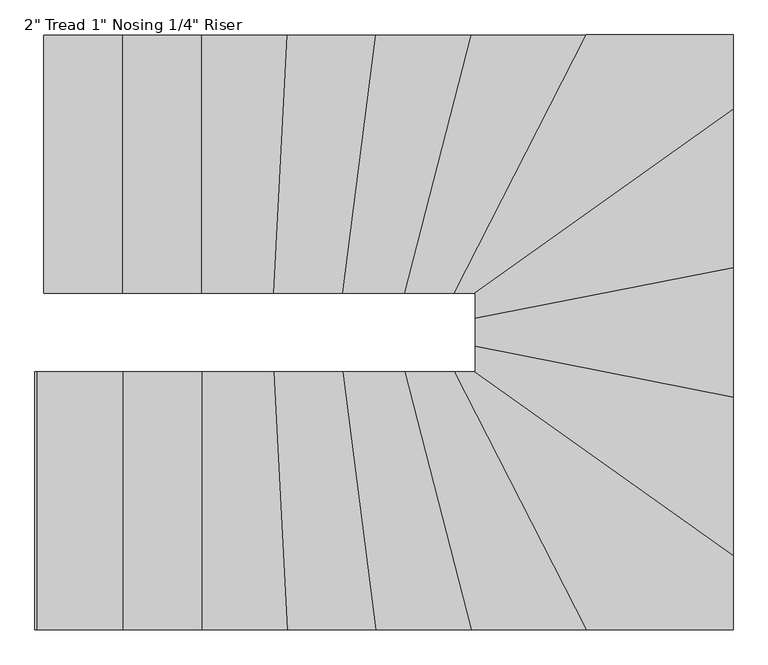
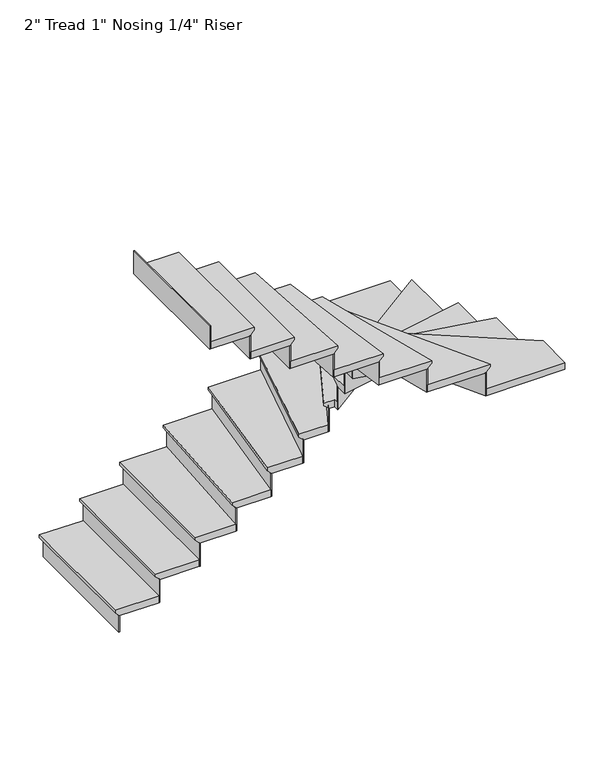
"""IFC4 building model written with IfcOpenShell, lengths in millimetres: stair flight geometry."""

from ifc_helpers import new_model, si_unit, origin, place, context, project, spatial, faceted_brep, source, transform, mapped, element, save


def stair_flight_bfa9ce03(model_context):
    return source(origin(), model_context, "Body", "Brep", [
        faceted_brep([(-5316.1183874, 7469.0787933, 150.2833333), (-5316.1183874, 7469.0787933, 169.3333333), (-5316.1183874, 8383.4787933, 169.3333333), (-5316.1183874, 8383.4787933, 150.2833333), (-5290.7183874, 7469.0787933, 124.8833333), (-5290.7183874, 8383.4787933, 124.8833333), (-5011.3183874, 7469.0787933, 169.3333333), (-5011.3183874, 8383.4787933, 169.3333333), (-5290.7183874, 8383.4787933, 118.5333333), (-5011.3183874, 8383.4787933, 118.5333333), (-5011.3183874, 7469.0787933, 118.5333333), (-5290.7183874, 7469.0787933, 118.5333333)], [[[0, 1, 2, 3]], [[4, 0, 3, 5]], [[2, 1, 6, 7]], [[8, 9, 10, 11]], [[2, 7, 9, 8, 5, 3]], [[8, 11, 4, 5]], [[6, 1, 0, 4, 11, 10]], [[7, 6, 10, 9]]]),
        faceted_brep([(-5290.7183874, 7469.0787933, 118.5333333), (-5290.7183874, 7469.0787933, 0.0), (-5284.3683874, 7469.0787933, 0.0), (-5284.3683874, 7469.0787933, 118.5333333), (-5290.7183874, 8383.4787933, 118.5333333), (-5284.3683874, 8383.4787933, 118.5333333), (-5284.3683874, 8383.4787933, 0.0), (-5290.7183874, 8383.4787933, 0.0)], [[[0, 1, 2, 3]], [[4, 5, 6, 7]], [[1, 0, 4, 7]], [[2, 1, 7, 6]], [[3, 2, 6, 5]], [[0, 3, 5, 4]]]),
        faceted_brep([(-5011.3183874, 7469.0787933, 287.8666667), (-5011.3183874, 7469.0787933, 118.5333333), (-5004.9683874, 7469.0787933, 118.5333333), (-5004.9683874, 7469.0787933, 287.8666667), (-5011.3183874, 8383.4787933, 287.8666667), (-5004.9683874, 8383.4787933, 287.8666667), (-5004.9683874, 8383.4787933, 118.5333333), (-5011.3183874, 8383.4787933, 118.5333333)], [[[0, 1, 2, 3]], [[4, 5, 6, 7]], [[1, 0, 4, 7]], [[2, 1, 7, 6]], [[3, 2, 6, 5]], [[0, 3, 5, 4]]]),
        faceted_brep([(-5036.7183874, 8383.4787933, 338.6666667), (-5036.7183874, 7469.0787933, 338.6666667), (-4731.9183874, 7469.0787933, 338.6666667), (-4731.9183874, 8383.4787933, 338.6666667), (-5011.3183874, 8383.4787933, 287.8666667), (-4731.9183874, 8383.4787933, 287.8666667), (-4731.9183874, 7469.0787933, 287.8666667), (-5011.3183874, 7469.0787933, 287.8666667), (-5011.3183874, 8383.4787933, 294.2166667), (-5036.7183874, 8383.4787933, 319.6166667), (-5011.3183874, 7469.0787933, 294.2166667), (-5036.7183874, 7469.0787933, 319.6166667)], [[[0, 1, 2, 3]], [[4, 5, 6, 7]], [[0, 3, 5, 4, 8, 9]], [[4, 7, 10, 8]], [[2, 1, 11, 10, 7, 6]], [[3, 2, 6, 5]], [[11, 1, 0, 9]], [[10, 11, 9, 8]]]),
        faceted_brep([(-4731.9183874, 7469.0787933, 457.2), (-4731.9183874, 7469.0787933, 287.8666667), (-4725.5683874, 7469.0787933, 287.8666667), (-4725.5683874, 7469.0787933, 457.2), (-4731.9183874, 8383.4787933, 457.2), (-4725.5683874, 8383.4787933, 457.2), (-4725.5683874, 8383.4787933, 287.8666667), (-4731.9183874, 8383.4787933, 287.8666667)], [[[0, 1, 2, 3]], [[4, 5, 6, 7]], [[1, 0, 4, 7]], [[2, 1, 7, 6]], [[3, 2, 6, 5]], [[0, 3, 5, 4]]]),
        faceted_brep([(-4757.3183874, 8383.4787933, 508.0), (-4757.3183874, 7469.0787933, 508.0), (-4476.2512259, 7469.0787933, 508.0), (-4428.7169555, 8383.4787933, 508.0), (-4731.9183874, 8383.4787933, 457.2), (-4428.7169555, 8383.4787933, 457.2), (-4476.2512259, 7469.0787933, 457.2), (-4731.9183874, 7469.0787933, 457.2), (-4731.9183874, 8383.4787933, 463.55), (-4757.3183874, 8383.4787933, 488.95), (-4731.9183874, 7469.0787933, 463.55), (-4757.3183874, 7469.0787933, 488.95)], [[[0, 1, 2, 3]], [[4, 5, 6, 7]], [[0, 3, 5, 4, 8, 9]], [[4, 7, 10, 8]], [[2, 1, 11, 10, 7, 6]], [[3, 2, 6, 5]], [[11, 1, 0, 9]], [[10, 11, 9, 8]]]),
        faceted_brep([(-4476.2512259, 7469.0787933, 626.5333333), (-4476.2512259, 7469.0787933, 457.2), (-4469.8926518, 7469.0787933, 457.2), (-4469.8926518, 7469.0787933, 626.5333333), (-4428.7169555, 8383.4787933, 626.5333333), (-4422.3583814, 8383.4787933, 626.5333333), (-4422.3583814, 8383.4787933, 457.2), (-4428.7169555, 8383.4787933, 457.2)], [[[0, 1, 2, 3]], [[4, 5, 6, 7]], [[1, 0, 4, 7]], [[2, 1, 7, 6]], [[3, 2, 6, 5]], [[0, 3, 5, 4]]]),
        faceted_brep([(-4454.1512522, 8383.4787933, 677.3333333), (-4501.6855226, 7469.0787933, 677.3333333), (-4232.0845261, 7469.0787933, 677.3333333), (-4113.7284745, 8383.4787933, 677.3333333), (-4428.7169555, 8383.4787933, 626.5333333), (-4113.7284745, 8383.4787933, 626.5333333), (-4232.0845261, 7469.0787933, 626.5333333), (-4476.2512259, 7469.0787933, 626.5333333), (-4428.7169555, 8383.4787933, 632.8833333), (-4454.1512522, 8383.4787933, 658.2833333), (-4476.2512259, 7469.0787933, 632.8833333), (-4501.6855226, 7469.0787933, 658.2833333)], [[[0, 1, 2, 3]], [[4, 5, 6, 7]], [[0, 3, 5, 4, 8, 9]], [[4, 7, 10, 8]], [[2, 1, 11, 10, 7, 6]], [[3, 2, 6, 5]], [[11, 1, 0, 9]], [[10, 11, 9, 8]]]),
        faceted_brep([(-4232.0845261, 7469.0787933, 795.8666667), (-4232.0845261, 7469.0787933, 626.5333333), (-4225.6815543, 7469.0787933, 626.5333333), (-4225.6815543, 7469.0787933, 795.8666667), (-4113.7284745, 8383.4787933, 795.8666667), (-4107.3255027, 8383.4787933, 795.8666667), (-4107.3255027, 8383.4787933, 626.5333333), (-4113.7284745, 8383.4787933, 626.5333333)], [[[0, 1, 2, 3]], [[4, 5, 6, 7]], [[1, 0, 4, 7]], [[2, 1, 7, 6]], [[3, 2, 6, 5]], [[0, 3, 5, 4]]]),
        faceted_brep([(-4139.3403616, 8383.4787933, 846.6666667), (-4257.6964132, 7469.0787933, 846.6666667), (-4010.4573036, 7469.0787933, 846.6666667), (-3775.3268562, 8383.4787933, 846.6666667), (-4113.7284745, 8383.4787933, 795.8666667), (-3775.3268562, 8383.4787933, 795.8666667), (-4010.4573036, 7469.0787933, 795.8666667), (-4232.0845261, 7469.0787933, 795.8666667), (-4113.7284745, 8383.4787933, 802.2166667), (-4139.3403616, 8383.4787933, 827.6166667), (-4232.0845261, 7469.0787933, 802.2166667), (-4257.6964132, 7469.0787933, 827.6166667)], [[[0, 1, 2, 3]], [[4, 5, 6, 7]], [[0, 3, 5, 4, 8, 9]], [[4, 7, 10, 8]], [[2, 1, 11, 10, 7, 6]], [[3, 2, 6, 5]], [[11, 1, 0, 9]], [[10, 11, 9, 8]]]),
        faceted_brep([(-4010.4573036, 7469.0787933, 965.2), (-4010.4573036, 7469.0787933, 795.8666667), (-4003.9007268, 7469.0787933, 795.8666667), (-4003.9007268, 7469.0787933, 965.2), (-3775.3268562, 8383.4787933, 965.2), (-3768.7702794, 8383.4787933, 965.2), (-3768.7702794, 8383.4787933, 795.8666667), (-3775.3268562, 8383.4787933, 795.8666667)], [[[0, 1, 2, 3]], [[4, 5, 6, 7]], [[1, 0, 4, 7]], [[2, 1, 7, 6]], [[3, 2, 6, 5]], [[0, 3, 5, 4]]]),
        faceted_brep([(-3801.5531637, 8383.4787933, 1016.0), (-4036.6836111, 7469.0787933, 1016.0), (-3834.1106676, 7469.0787933, 1016.0), (-3365.2860462, 8383.4787933, 1016.0), (-3775.3268562, 8383.4787933, 965.2), (-3365.2860462, 8383.4787933, 965.2), (-3834.1106676, 7469.0787933, 965.2), (-4010.4573036, 7469.0787933, 965.2), (-3775.3268562, 8383.4787933, 971.55), (-3801.5531637, 8383.4787933, 996.95), (-4010.4573036, 7469.0787933, 971.55), (-4036.6836111, 7469.0787933, 996.95)], [[[0, 1, 2, 3]], [[4, 5, 6, 7]], [[0, 3, 5, 4, 8, 9]], [[4, 7, 10, 8]], [[2, 1, 11, 10, 7, 6]], [[3, 2, 6, 5]], [[11, 1, 0, 9]], [[10, 11, 9, 8]]]),
        faceted_brep([(-3834.1106676, 7469.0787933, 1134.5333333), (-3834.1106676, 7469.0787933, 965.2), (-3826.9746844, 7469.0787933, 965.2), (-3826.9746844, 7469.0787933, 1134.5333333), (-3365.2860462, 8383.4787933, 1134.5333333), (-3358.1500631, 8383.4787933, 1134.5333333), (-3358.1500631, 8383.4787933, 965.2), (-3365.2860462, 8383.4787933, 965.2)], [[[0, 1, 2, 3]], [[4, 5, 6, 7]], [[1, 0, 4, 7]], [[2, 1, 7, 6]], [[3, 2, 6, 5]], [[0, 3, 5, 4]]]),
        faceted_brep([(-2873.9866955, 8089.7976596, 1185.3333333), (-2873.9866955, 8383.4787933, 1185.3333333), (-3393.8299788, 8383.4787933, 1185.3333333), (-3862.6546001, 7469.0787933, 1185.3333333), (-3788.3866955, 7469.0787933, 1185.3333333), (-3788.3866955, 7439.5237104, 1185.3333333), (-2873.9866955, 8383.4787933, 1134.5333333), (-2873.9866955, 8089.7976596, 1134.5333333), (-3788.3866955, 7439.5237104, 1134.5333333), (-3788.3866955, 7469.0787933, 1134.5333333), (-3834.1106676, 7469.0787933, 1134.5333333), (-3365.2860462, 8383.4787933, 1134.5333333), (-3365.2860462, 8383.4787933, 1140.8833333), (-3393.8299788, 8383.4787933, 1166.2833333), (-3834.1106676, 7469.0787933, 1140.8833333), (-3862.6546001, 7469.0787933, 1166.2833333)], [[[0, 1, 2, 3, 4, 5]], [[6, 7, 8, 9, 10, 11]], [[1, 0, 7, 6]], [[2, 1, 6, 11, 12, 13]], [[11, 10, 14, 12]], [[4, 3, 15, 14, 10, 9]], [[5, 4, 9, 8]], [[0, 5, 8, 7]], [[15, 3, 2, 13]], [[14, 15, 13, 12]]]),
        faceted_brep([(-3788.3866955, 7439.5237104, 1303.8666667), (-3788.3866955, 7439.5237104, 1134.5333333), (-3788.3866955, 7431.7317356, 1134.5333333), (-3788.3866955, 7431.7317356, 1303.8666667), (-2873.9866955, 8089.7976596, 1303.8666667), (-2873.9866955, 8082.0056848, 1303.8666667), (-2873.9866955, 8082.0056848, 1134.5333333), (-2873.9866955, 8089.7976596, 1134.5333333)], [[[0, 1, 2, 3]], [[4, 5, 6, 7]], [[1, 0, 4, 7]], [[2, 1, 7, 6]], [[3, 2, 6, 5]], [[0, 3, 5, 4]]]),
        faceted_brep([(-2873.9866955, 8120.9655588, 1354.6666667), (-3788.3866955, 7470.6916096, 1354.6666667), (-3788.3866955, 7353.0696234, 1354.6666667), (-2873.9866955, 7533.3104797, 1354.6666667), (-2873.9866955, 8089.7976596, 1303.8666667), (-2873.9866955, 7533.3104797, 1303.8666667), (-3788.3866955, 7353.0696234, 1303.8666667), (-3788.3866955, 7439.5237104, 1303.8666667), (-2873.9866955, 8089.7976596, 1310.2166667), (-2873.9866955, 8120.9655588, 1335.6166667), (-3788.3866955, 7439.5237104, 1310.2166667), (-3788.3866955, 7470.6916096, 1335.6166667)], [[[0, 1, 2, 3]], [[4, 5, 6, 7]], [[0, 3, 5, 4, 8, 9]], [[4, 7, 10, 8]], [[2, 1, 11, 10, 7, 6]], [[3, 2, 6, 5]], [[11, 1, 0, 9]], [[10, 11, 9, 8]]]),
        faceted_brep([(-3788.3866955, 7353.0696234, 1473.2), (-3788.3866955, 7353.0696234, 1303.8666667), (-3788.3866955, 7346.5974379, 1303.8666667), (-3788.3866955, 7346.5974379, 1473.2), (-2873.9866955, 7533.3104797, 1473.2), (-2873.9866955, 7526.8382943, 1473.2), (-2873.9866955, 7526.8382943, 1303.8666667), (-2873.9866955, 7533.3104797, 1303.8666667)], [[[0, 1, 2, 3]], [[4, 5, 6, 7]], [[1, 0, 4, 7]], [[2, 1, 7, 6]], [[3, 2, 6, 5]], [[0, 3, 5, 4]]]),
        faceted_brep([(-2873.9866955, 7559.1992214, 1524.0), (-3788.3866955, 7378.9583651, 1524.0), (-3788.3866955, 7253.9104797, 1524.0), (-2873.9866955, 7073.6696234, 1524.0), (-2873.9866955, 7533.3104797, 1473.2), (-2873.9866955, 7073.6696234, 1473.2), (-3788.3866955, 7253.9104797, 1473.2), (-3788.3866955, 7353.0696234, 1473.2), (-2873.9866955, 7533.3104797, 1479.55), (-2873.9866955, 7559.1992214, 1504.95), (-3788.3866955, 7353.0696234, 1479.55), (-3788.3866955, 7378.9583651, 1504.95)], [[[0, 1, 2, 3]], [[4, 5, 6, 7]], [[0, 3, 5, 4, 8, 9]], [[4, 7, 10, 8]], [[2, 1, 11, 10, 7, 6]], [[3, 2, 6, 5]], [[11, 1, 0, 9]], [[10, 11, 9, 8]]]),
        faceted_brep([(-3788.3866955, 7253.9104797, 1642.5333333), (-3788.3866955, 7253.9104797, 1473.2), (-3788.3866955, 7247.4382943, 1473.2), (-3788.3866955, 7247.4382943, 1642.5333333), (-2873.9866955, 7073.6696234, 1642.5333333), (-2873.9866955, 7067.1974379, 1642.5333333), (-2873.9866955, 7067.1974379, 1473.2), (-2873.9866955, 7073.6696234, 1473.2)], [[[0, 1, 2, 3]], [[4, 5, 6, 7]], [[1, 0, 4, 7]], [[2, 1, 7, 6]], [[3, 2, 6, 5]], [[0, 3, 5, 4]]]),
        faceted_brep([(-2873.9866955, 7099.5583651, 1693.3333333), (-3788.3866955, 7279.7992214, 1693.3333333), (-3788.3866955, 7189.6787933, 1693.3333333), (-3834.4821701, 7189.6787933, 1693.3333333), (-2873.9866955, 6506.6241286, 1693.3333333), (-2873.9866955, 7073.6696234, 1642.5333333), (-2873.9866955, 6506.6241286, 1642.5333333), (-3834.4821701, 7189.6787933, 1642.5333333), (-3788.3866955, 7189.6787933, 1642.5333333), (-3788.3866955, 7253.9104797, 1642.5333333), (-2873.9866955, 7073.6696234, 1648.8833333), (-2873.9866955, 7099.5583651, 1674.2833333), (-3788.3866955, 7253.9104797, 1648.8833333), (-3788.3866955, 7279.7992214, 1674.2833333)], [[[0, 1, 2, 3, 4]], [[5, 6, 7, 8, 9]], [[0, 4, 6, 5, 10, 11]], [[5, 9, 12, 10]], [[2, 1, 13, 12, 9, 8]], [[3, 2, 8, 7]], [[4, 3, 7, 6]], [[13, 1, 0, 11]], [[12, 13, 11, 10]]]),
        faceted_brep([(-3834.4821701, 7189.6787933, 1811.8666667), (-3834.4821701, 7189.6787933, 1642.5333333), (-3845.4390625, 7189.6787933, 1642.5333333), (-3845.4390625, 7189.6787933, 1811.8666667), (-2873.9866955, 6506.6241286, 1811.8666667), (-2873.9866955, 6498.8321538, 1811.8666667), (-2873.9866955, 6498.8321538, 1642.5333333), (-2873.9866955, 6506.6241286, 1642.5333333)], [[[0, 1, 2, 3]], [[4, 5, 6, 7]], [[1, 0, 4, 7]], [[2, 1, 7, 6]], [[3, 2, 6, 5]], [[0, 3, 5, 4]]]),
        faceted_brep([(-3422.3739113, 6275.2787933, 1862.6666667), (-2873.9866955, 6275.2787933, 1862.6666667), (-2873.9866955, 6537.7920278, 1862.6666667), (-3790.6546001, 7189.6787933, 1862.6666667), (-3891.1985326, 7189.6787933, 1862.6666667), (-2873.9866955, 6275.2787933, 1811.8666667), (-3422.3739113, 6275.2787933, 1811.8666667), (-3891.1985326, 7189.6787933, 1811.8666667), (-3834.4821701, 7189.6787933, 1811.8666667), (-2873.9866955, 6506.6241286, 1811.8666667), (-2873.9866955, 6506.6241286, 1818.2166667), (-2873.9866955, 6537.7920278, 1843.6166667), (-3834.4821701, 7189.6787933, 1818.2166667), (-3790.6546001, 7189.6787933, 1843.6166667)], [[[0, 1, 2, 3, 4]], [[5, 6, 7, 8, 9]], [[1, 0, 6, 5]], [[2, 1, 5, 9, 10, 11]], [[9, 8, 12, 10]], [[4, 3, 13, 12, 8, 7]], [[0, 4, 7, 6]], [[13, 3, 2, 11]], [[12, 13, 11, 10]]]),
        faceted_brep([(-3891.1985326, 7189.6787933, 1981.2), (-3891.1985326, 7189.6787933, 1811.8666667), (-3898.3345158, 7189.6787933, 1811.8666667), (-3898.3345158, 7189.6787933, 1981.2), (-3422.3739113, 6275.2787933, 1981.2), (-3429.5098944, 6275.2787933, 1981.2), (-3429.5098944, 6275.2787933, 1811.8666667), (-3422.3739113, 6275.2787933, 1811.8666667)], [[[0, 1, 2, 3]], [[4, 5, 6, 7]], [[1, 0, 4, 7]], [[2, 1, 7, 6]], [[3, 2, 6, 5]], [[0, 3, 5, 4]]]),
        faceted_brep([(-3393.8299788, 6275.2787933, 2032.0), (-3862.6546001, 7189.6787933, 2032.0), (-4062.9099186, 7189.6787933, 2032.0), (-3827.7794712, 6275.2787933, 2032.0), (-3422.3739113, 6275.2787933, 1981.2), (-3827.7794712, 6275.2787933, 1981.2), (-4062.9099186, 7189.6787933, 1981.2), (-3891.1985326, 7189.6787933, 1981.2), (-3422.3739113, 6275.2787933, 1987.55), (-3393.8299788, 6275.2787933, 2012.95), (-3891.1985326, 7189.6787933, 1987.55), (-3862.6546001, 7189.6787933, 2012.95)], [[[0, 1, 2, 3]], [[4, 5, 6, 7]], [[0, 3, 5, 4, 8, 9]], [[4, 7, 10, 8]], [[2, 1, 11, 10, 7, 6]], [[3, 2, 6, 5]], [[11, 1, 0, 9]], [[10, 11, 9, 8]]]),
        faceted_brep([(-4062.9099186, 7189.6787933, 2150.5333333), (-4062.9099186, 7189.6787933, 1981.2), (-4069.4664954, 7189.6787933, 1981.2), (-4069.4664954, 7189.6787933, 2150.5333333), (-3827.7794712, 6275.2787933, 2150.5333333), (-3834.336048, 6275.2787933, 2150.5333333), (-3834.336048, 6275.2787933, 1981.2), (-3827.7794712, 6275.2787933, 1981.2)], [[[0, 1, 2, 3]], [[4, 5, 6, 7]], [[1, 0, 4, 7]], [[2, 1, 7, 6]], [[3, 2, 6, 5]], [[0, 3, 5, 4]]]),
        faceted_brep([(-3801.5531637, 6275.2787933, 2201.3333333), (-4036.6836111, 7189.6787933, 2201.3333333), (-4283.3083003, 7189.6787933, 2201.3333333), (-4164.9522487, 6275.2787933, 2201.3333333), (-3827.7794712, 6275.2787933, 2150.5333333), (-4164.9522487, 6275.2787933, 2150.5333333), (-4283.3083003, 7189.6787933, 2150.5333333), (-4062.9099186, 7189.6787933, 2150.5333333), (-3827.7794712, 6275.2787933, 2156.8833333), (-3801.5531637, 6275.2787933, 2182.2833333), (-4062.9099186, 7189.6787933, 2156.8833333), (-4036.6836111, 7189.6787933, 2182.2833333)], [[[0, 1, 2, 3]], [[4, 5, 6, 7]], [[0, 3, 5, 4, 8, 9]], [[4, 7, 10, 8]], [[2, 1, 11, 10, 7, 6]], [[3, 2, 6, 5]], [[11, 1, 0, 9]], [[10, 11, 9, 8]]]),
        faceted_brep([(-4283.3083003, 7189.6787933, 2319.8666667), (-4283.3083003, 7189.6787933, 2150.5333333), (-4289.7112721, 7189.6787933, 2150.5333333), (-4289.7112721, 7189.6787933, 2319.8666667), (-4164.9522487, 6275.2787933, 2319.8666667), (-4171.3552205, 6275.2787933, 2319.8666667), (-4171.3552205, 6275.2787933, 2150.5333333), (-4164.9522487, 6275.2787933, 2150.5333333)], [[[0, 1, 2, 3]], [[4, 5, 6, 7]], [[1, 0, 4, 7]], [[2, 1, 7, 6]], [[3, 2, 6, 5]], [[0, 3, 5, 4]]]),
        faceted_brep([(-4139.3403616, 6275.2787933, 2370.6666667), (-4257.6964132, 7189.6787933, 2370.6666667), (-4527.1198193, 7189.6787933, 2370.6666667), (-4479.5855489, 6275.2787933, 2370.6666667), (-4164.9522487, 6275.2787933, 2319.8666667), (-4479.5855489, 6275.2787933, 2319.8666667), (-4527.1198193, 7189.6787933, 2319.8666667), (-4283.3083003, 7189.6787933, 2319.8666667), (-4164.9522487, 6275.2787933, 2326.2166667), (-4139.3403616, 6275.2787933, 2351.6166667), (-4283.3083003, 7189.6787933, 2326.2166667), (-4257.6964132, 7189.6787933, 2351.6166667)], [[[0, 1, 2, 3]], [[4, 5, 6, 7]], [[0, 3, 5, 4, 8, 9]], [[4, 7, 10, 8]], [[2, 1, 11, 10, 7, 6]], [[3, 2, 6, 5]], [[11, 1, 0, 9]], [[10, 11, 9, 8]]]),
        faceted_brep([(-4527.1198193, 7189.6787933, 2489.2), (-4527.1198193, 7189.6787933, 2319.8666667), (-4533.4783934, 7189.6787933, 2319.8666667), (-4533.4783934, 7189.6787933, 2489.2), (-4479.5855489, 6275.2787933, 2489.2), (-4485.944123, 6275.2787933, 2489.2), (-4485.944123, 6275.2787933, 2319.8666667), (-4479.5855489, 6275.2787933, 2319.8666667)], [[[0, 1, 2, 3]], [[4, 5, 6, 7]], [[1, 0, 4, 7]], [[2, 1, 7, 6]], [[3, 2, 6, 5]], [[0, 3, 5, 4]]]),
        faceted_brep([(-4454.1512522, 6275.2787933, 2540.0), (-4501.6855226, 7189.6787933, 2540.0), (-4782.7183874, 7189.6787933, 2540.0), (-4782.7183874, 6275.2787933, 2540.0), (-4479.5855489, 6275.2787933, 2489.2), (-4782.7183874, 6275.2787933, 2489.2), (-4782.7183874, 7189.6787933, 2489.2), (-4527.1198193, 7189.6787933, 2489.2), (-4479.5855489, 6275.2787933, 2495.55), (-4454.1512522, 6275.2787933, 2520.95), (-4527.1198193, 7189.6787933, 2495.55), (-4501.6855226, 7189.6787933, 2520.95)], [[[0, 1, 2, 3]], [[4, 5, 6, 7]], [[0, 3, 5, 4, 8, 9]], [[4, 7, 10, 8]], [[2, 1, 11, 10, 7, 6]], [[3, 2, 6, 5]], [[11, 1, 0, 9]], [[10, 11, 9, 8]]]),
        faceted_brep([(-4782.7183874, 7189.6787933, 2658.5333333), (-4782.7183874, 7189.6787933, 2489.2), (-4789.0683874, 7189.6787933, 2489.2), (-4789.0683874, 7189.6787933, 2658.5333333), (-4782.7183874, 6275.2787933, 2658.5333333), (-4789.0683874, 6275.2787933, 2658.5333333), (-4789.0683874, 6275.2787933, 2489.2), (-4782.7183874, 6275.2787933, 2489.2)], [[[0, 1, 2, 3]], [[4, 5, 6, 7]], [[1, 0, 4, 7]], [[2, 1, 7, 6]], [[3, 2, 6, 5]], [[0, 3, 5, 4]]]),
        faceted_brep([(-4757.3183874, 6275.2787933, 2709.3333333), (-4757.3183874, 7189.6787933, 2709.3333333), (-5062.1183874, 7189.6787933, 2709.3333333), (-5062.1183874, 6275.2787933, 2709.3333333), (-4782.7183874, 6275.2787933, 2658.5333333), (-5062.1183874, 6275.2787933, 2658.5333333), (-5062.1183874, 7189.6787933, 2658.5333333), (-4782.7183874, 7189.6787933, 2658.5333333), (-4782.7183874, 6275.2787933, 2664.8833333), (-4757.3183874, 6275.2787933, 2690.2833333), (-4782.7183874, 7189.6787933, 2664.8833333), (-4757.3183874, 7189.6787933, 2690.2833333)], [[[0, 1, 2, 3]], [[4, 5, 6, 7]], [[0, 3, 5, 4, 8, 9]], [[4, 7, 10, 8]], [[2, 1, 11, 10, 7, 6]], [[3, 2, 6, 5]], [[11, 1, 0, 9]], [[10, 11, 9, 8]]]),
        faceted_brep([(-5062.1183874, 7189.6787933, 2827.8666667), (-5062.1183874, 7189.6787933, 2658.5333333), (-5068.4683874, 7189.6787933, 2658.5333333), (-5068.4683874, 7189.6787933, 2827.8666667), (-5062.1183874, 6275.2787933, 2827.8666667), (-5068.4683874, 6275.2787933, 2827.8666667), (-5068.4683874, 6275.2787933, 2658.5333333), (-5062.1183874, 6275.2787933, 2658.5333333)], [[[0, 1, 2, 3]], [[4, 5, 6, 7]], [[1, 0, 4, 7]], [[2, 1, 7, 6]], [[3, 2, 6, 5]], [[0, 3, 5, 4]]]),
        faceted_brep([(-5341.5183874, 7189.6787933, 2997.2), (-5341.5183874, 7189.6787933, 2827.8666667), (-5347.8683874, 7189.6787933, 2827.8666667), (-5347.8683874, 7189.6787933, 2997.2), (-5341.5183874, 6275.2787933, 2997.2), (-5347.8683874, 6275.2787933, 2997.2), (-5347.8683874, 6275.2787933, 2827.8666667), (-5341.5183874, 6275.2787933, 2827.8666667)], [[[0, 1, 2, 3]], [[4, 5, 6, 7]], [[1, 0, 4, 7]], [[2, 1, 7, 6]], [[3, 2, 6, 5]], [[0, 3, 5, 4]]]),
        faceted_brep([(-5036.7183874, 6275.2787933, 2878.6666667), (-5036.7183874, 7189.6787933, 2878.6666667), (-5341.5183874, 7189.6787933, 2878.6666667), (-5341.5183874, 6275.2787933, 2878.6666667), (-5062.1183874, 6275.2787933, 2827.8666667), (-5341.5183874, 6275.2787933, 2827.8666667), (-5341.5183874, 7189.6787933, 2827.8666667), (-5062.1183874, 7189.6787933, 2827.8666667), (-5062.1183874, 6275.2787933, 2834.2166667), (-5036.7183874, 6275.2787933, 2859.6166667), (-5062.1183874, 7189.6787933, 2834.2166667), (-5036.7183874, 7189.6787933, 2859.6166667)], [[[0, 1, 2, 3]], [[4, 5, 6, 7]], [[0, 3, 5, 4, 8, 9]], [[4, 7, 10, 8]], [[2, 1, 11, 10, 7, 6]], [[3, 2, 6, 5]], [[11, 1, 0, 9]], [[10, 11, 9, 8]]]),
    ])


if __name__ == "__main__":
    model = new_model("IFC4")
    model_context = context("Model", 3, world=origin())
    ifc_project = project(units=[si_unit("LENGTHUNIT", "METRE", prefix="MILLI")], contexts=[model_context])
    site = spatial("IfcSite", under=ifc_project)
    building = spatial("IfcBuilding", under=site)
    placement = place(None, origin())
    stair_flight_shape = stair_flight_bfa9ce03(model_context)
    element("IfcStairFlight", 1, ObjectType="2\" Tread 1\" Nosing 1/4\" Riser", at=placement, inside=building, context=model_context, shape_type="MappedRepresentation", body=[
        mapped(stair_flight_shape, transform((0.0, 0.0, 0.0), x_axis=(1.0, 0.0, 0.0), y_axis=(0.0, 1.0, 0.0), z_axis=(0.0, 0.0, 1.0))),
    ])
    save(model, "model.ifc")
